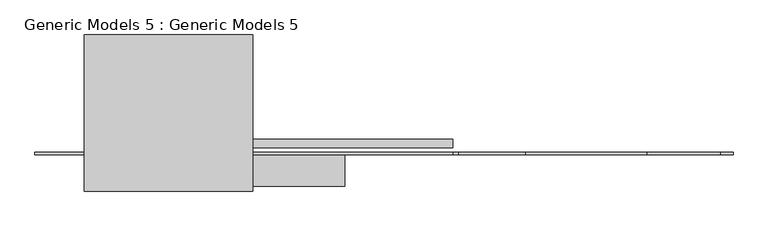
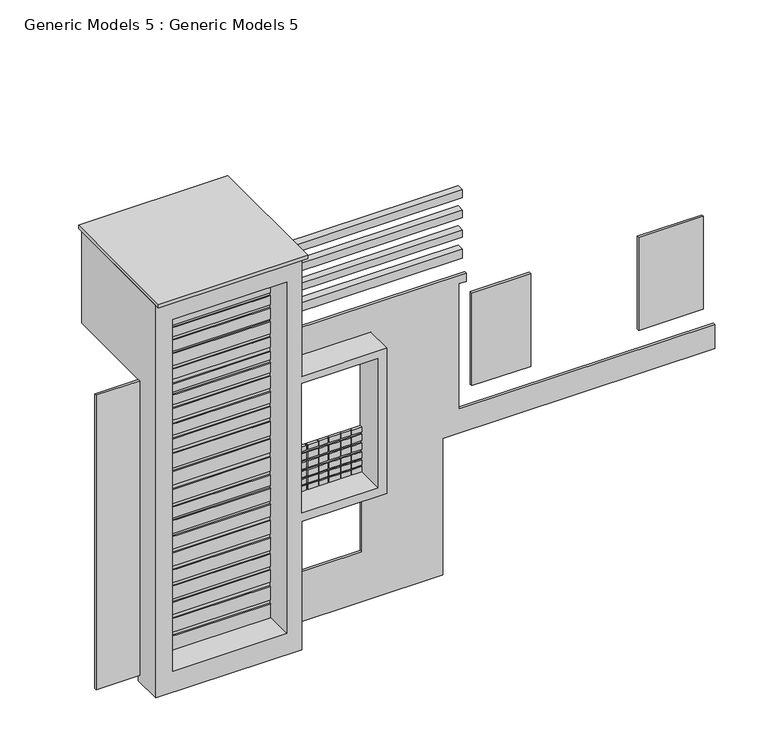
"""IFC4 building model written with IfcOpenShell, lengths in millimetres: proxy geometry, Generic Models 5 : Generic Models 5."""

from ifc_helpers import new_model, si_unit, frame, origin, place, context, project, spatial, polyline, outline, extrude, faceted_brep, source, transform, mapped, element, save


def generic_models_5_generic_models_5_751a22c3(model_context):
    return source(origin(), model_context, "Body", "SolidModel", [
        extrude(outline(polyline([(-4031.0859258, -11851.8777232), (-5326.4859258, -11851.8777232), (-5326.4859258, -11801.0777232), (-4031.0859258, -11801.0777232), (-4031.0859258, -11851.8777232)])), frame((0.0, 0.0, 3959.8880455), z_axis=(0.0, 0.0, 1.0), x_axis=(1.0, 0.0, 0.0)), (0.0, 0.0, 1.0), 1974.0451783),
        extrude(outline(polyline([(-7498.1859258, -11851.8777232), (-8679.2859258, -11851.8777232), (-8679.2859258, -11801.0777232), (-7498.1859258, -11801.0777232), (-7498.1859258, -11851.8777232)])), frame((0.0, 0.0, 3961.5542172), z_axis=(0.0, 0.0, 1.0), x_axis=(1.0, 0.0, 0.0)), (0.0, 0.0, 1.0), 1972.3790066),
        faceted_brep([(-12413.0859258, -11851.8777232, 3860.2469154), (-12413.0859258, -11851.8777232, 3758.0237467), (-12212.1386934, -11851.8777232, 3758.0237467), (-12212.1386934, -11851.8777232, 3860.2469154), (-12413.0859258, -11851.8777232, 3705.6018862), (-12413.0859258, -11851.8777232, 3567.9945022), (-12212.1386934, -11851.8777232, 3567.9945022), (-12212.1386934, -11851.8777232, 3705.6018862), (-12413.0859258, -11851.8777232, 3518.8490079), (-12413.0859258, -11851.8777232, 3383.7067756), (-12212.1386934, -11851.8777232, 3383.7067756), (-12212.1386934, -11851.8777232, 3518.8490079), (-12413.0859258, -11851.8777232, 3332.0961296), (-12413.0859258, -11851.8777232, 3204.3178444), (-12212.1386934, -11851.8777232, 3204.3178444), (-12212.1386934, -11851.8777232, 3332.0961296), (-12413.0859258, -11851.8777232, 3015.7193284), (-12413.0859258, -11851.8777232, 2907.1666358), (-12212.1386934, -11851.8777232, 2907.1666358), (-12212.1386934, -11851.8777232, 3015.7193284), (-12413.0859258, -11851.8777232, 3163.365824), (-12413.0859258, -11851.8777232, 3048.0), (-12212.1386934, -11851.8777232, 3048.0), (-12212.1386934, -11851.8777232, 3163.365824), (-10889.0859258, -11851.8777232, 3758.0237467), (-10889.0859258, -11851.8777232, 3860.2469154), (-11089.7671408, -11851.8777232, 3860.2469154), (-11089.7671408, -11851.8777232, 3758.0237467), (-10889.0859258, -11851.8777232, 3567.9945022), (-10889.0859258, -11851.8777232, 3705.6018862), (-11089.7671408, -11851.8777232, 3705.6018862), (-11089.7671408, -11851.8777232, 3567.9945022), (-10889.0859258, -11851.8777232, 3383.7067756), (-10889.0859258, -11851.8777232, 3518.8490079), (-11089.7671408, -11851.8777232, 3518.8490079), (-11089.7671408, -11851.8777232, 3383.7067756), (-10889.0859258, -11851.8777232, 3204.3178444), (-10889.0859258, -11851.8777232, 3332.0961296), (-11089.7671408, -11851.8777232, 3332.0961296), (-11089.7671408, -11851.8777232, 3204.3178444), (-10889.0859258, -11851.8777232, 2907.1666358), (-10889.0859258, -11851.8777232, 3015.7193284), (-11089.7671408, -11851.8777232, 3015.7193284), (-11089.7671408, -11851.8777232, 2907.1666358), (-10889.0859258, -11851.8777232, 3048.0), (-10889.0859258, -11851.8777232, 3163.365824), (-11089.7671408, -11851.8777232, 3163.365824), (-11089.7671408, -11851.8777232, 3048.0), (-11318.1191266, -11851.8777232, 3860.2469154), (-11542.1625843, -11851.8777232, 3860.2469154), (-11542.1625843, -11851.8777232, 3758.0237467), (-11318.1191266, -11851.8777232, 3758.0237467), (-11107.0012529, -11851.8777232, 3860.2469154), (-11300.8850144, -11851.8777232, 3860.2469154), (-11300.8850144, -11851.8777232, 3758.0237467), (-11107.0012529, -11851.8777232, 3758.0237467), (-11568.0137525, -11851.8777232, 3860.2469154), (-11742.5091378, -11851.8777232, 3860.2469154), (-11742.5091378, -11851.8777232, 3758.0237467), (-11568.0137525, -11851.8777232, 3758.0237467), (-11766.206042, -11851.8777232, 3860.2469154), (-11977.3239156, -11851.8777232, 3860.2469154), (-11977.3239156, -11851.8777232, 3758.0237467), (-11766.206042, -11851.8777232, 3758.0237467), (-12005.3293478, -11851.8777232, 3860.2469154), (-12192.7503172, -11851.8777232, 3860.2469154), (-12192.7503172, -11851.8777232, 3758.0237467), (-12005.3293478, -11851.8777232, 3758.0237467), (-11542.1625843, -11851.8777232, 2907.1666358), (-11318.1191266, -11851.8777232, 2907.1666358), (-11318.1191266, -11851.8777232, 3015.7193284), (-11542.1625843, -11851.8777232, 3015.7193284), (-11300.8850144, -11851.8777232, 2907.1666358), (-11107.0012529, -11851.8777232, 2907.1666358), (-11107.0012529, -11851.8777232, 3015.7193284), (-11300.8850144, -11851.8777232, 3015.7193284), (-11742.5091378, -11851.8777232, 2907.1666358), (-11568.0137525, -11851.8777232, 2907.1666358), (-11568.0137525, -11851.8777232, 3015.7193284), (-11742.5091378, -11851.8777232, 3015.7193284), (-11977.3239156, -11851.8777232, 2907.1666358), (-11766.206042, -11851.8777232, 2907.1666358), (-11766.206042, -11851.8777232, 3015.7193284), (-11977.3239156, -11851.8777232, 3015.7193284), (-12192.7503172, -11851.8777232, 2907.1666358), (-12005.3293478, -11851.8777232, 2907.1666358), (-12005.3293478, -11851.8777232, 3015.7193284), (-12192.7503172, -11851.8777232, 3015.7193284), (-11542.1625843, -11851.8777232, 3567.9945022), (-11318.1191266, -11851.8777232, 3567.9945022), (-11318.1191266, -11851.8777232, 3705.6018862), (-11542.1625843, -11851.8777232, 3705.6018862), (-11300.8850144, -11851.8777232, 3567.9945022), (-11107.0012529, -11851.8777232, 3567.9945022), (-11107.0012529, -11851.8777232, 3705.6018862), (-11300.8850144, -11851.8777232, 3705.6018862), (-11742.5091378, -11851.8777232, 3567.9945022), (-11568.0137525, -11851.8777232, 3567.9945022), (-11568.0137525, -11851.8777232, 3705.6018862), (-11742.5091378, -11851.8777232, 3705.6018862), (-11977.3239156, -11851.8777232, 3567.9945022), (-11766.206042, -11851.8777232, 3567.9945022), (-11766.206042, -11851.8777232, 3705.6018862), (-11977.3239156, -11851.8777232, 3705.6018862), (-12192.7503172, -11851.8777232, 3567.9945022), (-12005.3293478, -11851.8777232, 3567.9945022), (-12005.3293478, -11851.8777232, 3705.6018862), (-12192.7503172, -11851.8777232, 3705.6018862), (-11542.1625843, -11851.8777232, 3383.7067756), (-11318.1191266, -11851.8777232, 3383.7067756), (-11318.1191266, -11851.8777232, 3518.8490079), (-11542.1625843, -11851.8777232, 3518.8490079), (-11300.8850144, -11851.8777232, 3383.7067756), (-11107.0012529, -11851.8777232, 3383.7067756), (-11107.0012529, -11851.8777232, 3518.8490079), (-11300.8850144, -11851.8777232, 3518.8490079), (-11742.5091378, -11851.8777232, 3383.7067756), (-11568.0137525, -11851.8777232, 3383.7067756), (-11568.0137525, -11851.8777232, 3518.8490079), (-11742.5091378, -11851.8777232, 3518.8490079), (-11977.3239156, -11851.8777232, 3383.7067756), (-11766.206042, -11851.8777232, 3383.7067756), (-11766.206042, -11851.8777232, 3518.8490079), (-11977.3239156, -11851.8777232, 3518.8490079), (-12192.7503172, -11851.8777232, 3383.7067756), (-12005.3293478, -11851.8777232, 3383.7067756), (-12005.3293478, -11851.8777232, 3518.8490079), (-12192.7503172, -11851.8777232, 3518.8490079), (-11542.1625843, -11851.8777232, 3204.3178444), (-11318.1191266, -11851.8777232, 3204.3178444), (-11318.1191266, -11851.8777232, 3332.0961296), (-11542.1625843, -11851.8777232, 3332.0961296), (-11300.8850144, -11851.8777232, 3204.3178444), (-11107.0012529, -11851.8777232, 3204.3178444), (-11107.0012529, -11851.8777232, 3332.0961296), (-11300.8850144, -11851.8777232, 3332.0961296), (-11742.5091378, -11851.8777232, 3204.3178444), (-11568.0137525, -11851.8777232, 3204.3178444), (-11568.0137525, -11851.8777232, 3332.0961296), (-11742.5091378, -11851.8777232, 3332.0961296), (-11977.3239156, -11851.8777232, 3204.3178444), (-11766.206042, -11851.8777232, 3204.3178444), (-11766.206042, -11851.8777232, 3332.0961296), (-11977.3239156, -11851.8777232, 3332.0961296), (-12192.7503172, -11851.8777232, 3204.3178444), (-12005.3293478, -11851.8777232, 3204.3178444), (-12005.3293478, -11851.8777232, 3332.0961296), (-12192.7503172, -11851.8777232, 3332.0961296), (-11542.1625843, -11851.8777232, 3048.0), (-11318.1191266, -11851.8777232, 3048.0), (-11318.1191266, -11851.8777232, 3163.365824), (-11542.1625843, -11851.8777232, 3163.365824), (-11300.8850144, -11851.8777232, 3048.0), (-11107.0012529, -11851.8777232, 3048.0), (-11107.0012529, -11851.8777232, 3163.365824), (-11300.8850144, -11851.8777232, 3163.365824), (-11742.5091378, -11851.8777232, 3048.0), (-11568.0137525, -11851.8777232, 3048.0), (-11568.0137525, -11851.8777232, 3163.365824), (-11742.5091378, -11851.8777232, 3163.365824), (-11977.3239156, -11851.8777232, 3048.0), (-11766.206042, -11851.8777232, 3048.0), (-11766.206042, -11851.8777232, 3163.365824), (-11977.3239156, -11851.8777232, 3163.365824), (-12192.7503172, -11851.8777232, 3048.0), (-12005.3293478, -11851.8777232, 3048.0), (-12005.3293478, -11851.8777232, 3163.365824), (-12192.7503172, -11851.8777232, 3163.365824), (-10889.0859258, -11801.0777232, 3860.2469154), (-10889.0859258, -11801.0777232, 2907.1666358), (-12413.0859258, -11801.0777232, 2907.1666358), (-12413.0859258, -11801.0777232, 3860.2469154), (-12212.1386934, -11826.4777232, 3860.2469154), (-12192.7503172, -11826.4777232, 3860.2469154), (-12005.3293478, -11826.4777232, 3860.2469154), (-11977.3239156, -11826.4777232, 3860.2469154), (-11766.206042, -11826.4777232, 3860.2469154), (-11742.5091378, -11826.4777232, 3860.2469154), (-11568.0137525, -11826.4777232, 3860.2469154), (-11542.1625843, -11826.4777232, 3860.2469154), (-11318.1191266, -11826.4777232, 3860.2469154), (-11300.8850144, -11826.4777232, 3860.2469154), (-11107.0012529, -11826.4777232, 3860.2469154), (-11089.7671408, -11826.4777232, 3860.2469154), (-12413.0859258, -11826.4777232, 3015.7193284), (-12413.0859258, -11826.4777232, 3048.0), (-12413.0859258, -11826.4777232, 3163.365824), (-12413.0859258, -11826.4777232, 3204.3178444), (-12413.0859258, -11826.4777232, 3332.0961296), (-12413.0859258, -11826.4777232, 3383.7067756), (-12413.0859258, -11826.4777232, 3518.8490079), (-12413.0859258, -11826.4777232, 3567.9945022), (-12413.0859258, -11826.4777232, 3705.6018862), (-12413.0859258, -11826.4777232, 3758.0237467), (-11089.7671408, -11826.4777232, 2907.1666358), (-11107.0012529, -11826.4777232, 2907.1666358), (-11300.8850144, -11826.4777232, 2907.1666358), (-11318.1191266, -11826.4777232, 2907.1666358), (-11542.1625843, -11826.4777232, 2907.1666358), (-11568.0137525, -11826.4777232, 2907.1666358), (-11742.5091378, -11826.4777232, 2907.1666358), (-11766.206042, -11826.4777232, 2907.1666358), (-11977.3239156, -11826.4777232, 2907.1666358), (-12005.3293478, -11826.4777232, 2907.1666358), (-12192.7503172, -11826.4777232, 2907.1666358), (-12212.1386934, -11826.4777232, 2907.1666358), (-10889.0859258, -11826.4777232, 3758.0237467), (-10889.0859258, -11826.4777232, 3705.6018862), (-10889.0859258, -11826.4777232, 3567.9945022), (-10889.0859258, -11826.4777232, 3518.8490079), (-10889.0859258, -11826.4777232, 3383.7067756), (-10889.0859258, -11826.4777232, 3332.0961296), (-10889.0859258, -11826.4777232, 3204.3178444), (-10889.0859258, -11826.4777232, 3163.365824), (-10889.0859258, -11826.4777232, 3048.0), (-10889.0859258, -11826.4777232, 3015.7193284), (-12212.1386934, -11826.4777232, 3705.6018862), (-12212.1386934, -11826.4777232, 3567.9945022), (-12212.1386934, -11826.4777232, 3518.8490079), (-12212.1386934, -11826.4777232, 3383.7067756), (-12212.1386934, -11826.4777232, 3332.0961296), (-12212.1386934, -11826.4777232, 3204.3178444), (-12212.1386934, -11826.4777232, 3163.365824), (-12212.1386934, -11826.4777232, 3048.0), (-12212.1386934, -11826.4777232, 3015.7193284), (-12192.7503172, -11826.4777232, 3015.7193284), (-12005.3293478, -11826.4777232, 3015.7193284), (-11977.3239156, -11826.4777232, 3015.7193284), (-11766.206042, -11826.4777232, 3015.7193284), (-11742.5091378, -11826.4777232, 3015.7193284), (-11568.0137525, -11826.4777232, 3015.7193284), (-11542.1625843, -11826.4777232, 3015.7193284), (-11318.1191266, -11826.4777232, 3015.7193284), (-11300.8850144, -11826.4777232, 3015.7193284), (-11107.0012529, -11826.4777232, 3015.7193284), (-11089.7671408, -11826.4777232, 3015.7193284), (-11089.7671408, -11826.4777232, 3048.0), (-11089.7671408, -11826.4777232, 3163.365824), (-11089.7671408, -11826.4777232, 3204.3178444), (-11089.7671408, -11826.4777232, 3332.0961296), (-11089.7671408, -11826.4777232, 3383.7067756), (-11089.7671408, -11826.4777232, 3518.8490079), (-11089.7671408, -11826.4777232, 3567.9945022), (-11089.7671408, -11826.4777232, 3705.6018862), (-11089.7671408, -11826.4777232, 3758.0237467), (-11107.0012529, -11826.4777232, 3758.0237467), (-11300.8850144, -11826.4777232, 3758.0237467), (-11318.1191266, -11826.4777232, 3758.0237467), (-11542.1625843, -11826.4777232, 3758.0237467), (-11568.0137525, -11826.4777232, 3758.0237467), (-11742.5091378, -11826.4777232, 3758.0237467), (-11766.206042, -11826.4777232, 3758.0237467), (-11977.3239156, -11826.4777232, 3758.0237467), (-12005.3293478, -11826.4777232, 3758.0237467), (-12192.7503172, -11826.4777232, 3758.0237467), (-12212.1386934, -11826.4777232, 3758.0237467), (-11542.1625843, -11826.4777232, 3705.6018862), (-11318.1191266, -11826.4777232, 3705.6018862), (-11318.1191266, -11826.4777232, 3567.9945022), (-11542.1625843, -11826.4777232, 3567.9945022), (-11300.8850144, -11826.4777232, 3705.6018862), (-11107.0012529, -11826.4777232, 3705.6018862), (-11107.0012529, -11826.4777232, 3567.9945022), (-11300.8850144, -11826.4777232, 3567.9945022), (-11742.5091378, -11826.4777232, 3705.6018862), (-11568.0137525, -11826.4777232, 3705.6018862), (-11568.0137525, -11826.4777232, 3567.9945022), (-11742.5091378, -11826.4777232, 3567.9945022), (-11977.3239156, -11826.4777232, 3705.6018862), (-11766.206042, -11826.4777232, 3705.6018862), (-11766.206042, -11826.4777232, 3567.9945022), (-11977.3239156, -11826.4777232, 3567.9945022), (-12192.7503172, -11826.4777232, 3705.6018862), (-12005.3293478, -11826.4777232, 3705.6018862), (-12005.3293478, -11826.4777232, 3567.9945022), (-12192.7503172, -11826.4777232, 3567.9945022), (-11542.1625843, -11826.4777232, 3518.8490079), (-11318.1191266, -11826.4777232, 3518.8490079), (-11318.1191266, -11826.4777232, 3383.7067756), (-11542.1625843, -11826.4777232, 3383.7067756), (-11300.8850144, -11826.4777232, 3518.8490079), (-11107.0012529, -11826.4777232, 3518.8490079), (-11107.0012529, -11826.4777232, 3383.7067756), (-11300.8850144, -11826.4777232, 3383.7067756), (-11742.5091378, -11826.4777232, 3518.8490079), (-11568.0137525, -11826.4777232, 3518.8490079), (-11568.0137525, -11826.4777232, 3383.7067756), (-11742.5091378, -11826.4777232, 3383.7067756), (-11977.3239156, -11826.4777232, 3518.8490079), (-11766.206042, -11826.4777232, 3518.8490079), (-11766.206042, -11826.4777232, 3383.7067756), (-11977.3239156, -11826.4777232, 3383.7067756), (-12192.7503172, -11826.4777232, 3518.8490079), (-12005.3293478, -11826.4777232, 3518.8490079), (-12005.3293478, -11826.4777232, 3383.7067756), (-12192.7503172, -11826.4777232, 3383.7067756), (-11542.1625843, -11826.4777232, 3332.0961296), (-11318.1191266, -11826.4777232, 3332.0961296), (-11318.1191266, -11826.4777232, 3204.3178444), (-11542.1625843, -11826.4777232, 3204.3178444), (-11300.8850144, -11826.4777232, 3332.0961296), (-11107.0012529, -11826.4777232, 3332.0961296), (-11107.0012529, -11826.4777232, 3204.3178444), (-11300.8850144, -11826.4777232, 3204.3178444), (-11742.5091378, -11826.4777232, 3332.0961296), (-11568.0137525, -11826.4777232, 3332.0961296), (-11568.0137525, -11826.4777232, 3204.3178444), (-11742.5091378, -11826.4777232, 3204.3178444), (-11977.3239156, -11826.4777232, 3332.0961296), (-11766.206042, -11826.4777232, 3332.0961296), (-11766.206042, -11826.4777232, 3204.3178444), (-11977.3239156, -11826.4777232, 3204.3178444), (-12192.7503172, -11826.4777232, 3332.0961296), (-12005.3293478, -11826.4777232, 3332.0961296), (-12005.3293478, -11826.4777232, 3204.3178444), (-12192.7503172, -11826.4777232, 3204.3178444), (-11542.1625843, -11826.4777232, 3163.365824), (-11318.1191266, -11826.4777232, 3163.365824), (-11318.1191266, -11826.4777232, 3048.0), (-11542.1625843, -11826.4777232, 3048.0), (-11300.8850144, -11826.4777232, 3163.365824), (-11107.0012529, -11826.4777232, 3163.365824), (-11107.0012529, -11826.4777232, 3048.0), (-11300.8850144, -11826.4777232, 3048.0), (-11742.5091378, -11826.4777232, 3163.365824), (-11568.0137525, -11826.4777232, 3163.365824), (-11568.0137525, -11826.4777232, 3048.0), (-11742.5091378, -11826.4777232, 3048.0), (-11977.3239156, -11826.4777232, 3163.365824), (-11766.206042, -11826.4777232, 3163.365824), (-11766.206042, -11826.4777232, 3048.0), (-11977.3239156, -11826.4777232, 3048.0), (-12192.7503172, -11826.4777232, 3163.365824), (-12005.3293478, -11826.4777232, 3163.365824), (-12005.3293478, -11826.4777232, 3048.0), (-12192.7503172, -11826.4777232, 3048.0)], [[[0, 1, 2, 3]], [[4, 5, 6, 7]], [[8, 9, 10, 11]], [[12, 13, 14, 15]], [[16, 17, 18, 19]], [[20, 21, 22, 23]], [[24, 25, 26, 27]], [[28, 29, 30, 31]], [[32, 33, 34, 35]], [[36, 37, 38, 39]], [[40, 41, 42, 43]], [[44, 45, 46, 47]], [[48, 49, 50, 51]], [[52, 53, 54, 55]], [[56, 57, 58, 59]], [[60, 61, 62, 63]], [[64, 65, 66, 67]], [[68, 69, 70, 71]], [[72, 73, 74, 75]], [[76, 77, 78, 79]], [[80, 81, 82, 83]], [[84, 85, 86, 87]], [[88, 89, 90, 91]], [[92, 93, 94, 95]], [[96, 97, 98, 99]], [[100, 101, 102, 103]], [[104, 105, 106, 107]], [[108, 109, 110, 111]], [[112, 113, 114, 115]], [[116, 117, 118, 119]], [[120, 121, 122, 123]], [[124, 125, 126, 127]], [[128, 129, 130, 131]], [[132, 133, 134, 135]], [[136, 137, 138, 139]], [[140, 141, 142, 143]], [[144, 145, 146, 147]], [[148, 149, 150, 151]], [[152, 153, 154, 155]], [[156, 157, 158, 159]], [[160, 161, 162, 163]], [[164, 165, 166, 167]], [[168, 169, 170, 171]], [[168, 171, 0, 3, 172, 173, 65, 64, 174, 175, 61, 60, 176, 177, 57, 56, 178, 179, 49, 48, 180, 181, 53, 52, 182, 183, 26, 25]], [[171, 170, 17, 16, 184, 185, 21, 20, 186, 187, 13, 12, 188, 189, 9, 8, 190, 191, 5, 4, 192, 193, 1, 0]], [[170, 169, 40, 43, 194, 195, 73, 72, 196, 197, 69, 68, 198, 199, 77, 76, 200, 201, 81, 80, 202, 203, 85, 84, 204, 205, 18, 17]], [[169, 168, 25, 24, 206, 207, 29, 28, 208, 209, 33, 32, 210, 211, 37, 36, 212, 213, 45, 44, 214, 215, 41, 40]], [[193, 192, 216, 217, 191, 190, 218, 219, 189, 188, 220, 221, 187, 186, 222, 223, 185, 184, 224, 205, 204, 225, 226, 203, 202, 227, 228, 201, 200, 229, 230, 199, 198, 231, 232, 197, 196, 233, 234, 195, 194, 235, 215, 214, 236, 237, 213, 212, 238, 239, 211, 210, 240, 241, 209, 208, 242, 243, 207, 206, 244, 183, 182, 245, 246, 181, 180, 247, 248, 179, 178, 249, 250, 177, 176, 251, 252, 175, 174, 253, 254, 173, 172, 255], [256, 257, 258, 259], [260, 261, 262, 263], [264, 265, 266, 267], [268, 269, 270, 271], [272, 273, 274, 275], [276, 277, 278, 279], [280, 281, 282, 283], [284, 285, 286, 287], [288, 289, 290, 291], [292, 293, 294, 295], [296, 297, 298, 299], [300, 301, 302, 303], [304, 305, 306, 307], [308, 309, 310, 311], [312, 313, 314, 315], [316, 317, 318, 319], [320, 321, 322, 323], [324, 325, 326, 327], [328, 329, 330, 331], [332, 333, 334, 335]], [[91, 90, 257, 256]], [[95, 94, 261, 260]], [[99, 98, 265, 264]], [[103, 102, 269, 268]], [[107, 106, 273, 272]], [[192, 4, 7, 216]], [[29, 207, 243, 30]], [[51, 50, 248, 247]], [[55, 54, 246, 245]], [[59, 58, 250, 249]], [[63, 62, 252, 251]], [[67, 66, 254, 253]], [[1, 193, 255, 2]], [[206, 24, 27, 244]], [[111, 110, 277, 276]], [[115, 114, 281, 280]], [[119, 118, 285, 284]], [[123, 122, 289, 288]], [[127, 126, 293, 292]], [[190, 8, 11, 218]], [[33, 209, 241, 34]], [[89, 88, 259, 258]], [[93, 92, 263, 262]], [[97, 96, 267, 266]], [[101, 100, 271, 270]], [[105, 104, 275, 274]], [[5, 191, 217, 6]], [[208, 28, 31, 242]], [[131, 130, 297, 296]], [[135, 134, 301, 300]], [[139, 138, 305, 304]], [[143, 142, 309, 308]], [[147, 146, 313, 312]], [[188, 12, 15, 220]], [[37, 211, 239, 38]], [[109, 108, 279, 278]], [[113, 112, 283, 282]], [[117, 116, 287, 286]], [[121, 120, 291, 290]], [[125, 124, 295, 294]], [[9, 189, 219, 10]], [[210, 32, 35, 240]], [[151, 150, 317, 316]], [[155, 154, 321, 320]], [[159, 158, 325, 324]], [[163, 162, 329, 328]], [[167, 166, 333, 332]], [[186, 20, 23, 222]], [[45, 213, 237, 46]], [[129, 128, 299, 298]], [[133, 132, 303, 302]], [[137, 136, 307, 306]], [[141, 140, 311, 310]], [[145, 144, 315, 314]], [[13, 187, 221, 14]], [[212, 36, 39, 238]], [[71, 70, 232, 231]], [[75, 74, 234, 233]], [[79, 78, 230, 229]], [[83, 82, 228, 227]], [[87, 86, 226, 225]], [[184, 16, 19, 224]], [[41, 215, 235, 42]], [[149, 148, 319, 318]], [[153, 152, 323, 322]], [[157, 156, 327, 326]], [[161, 160, 331, 330]], [[165, 164, 335, 334]], [[21, 185, 223, 22]], [[214, 44, 47, 236]], [[231, 198, 68, 71]], [[179, 248, 50, 49]], [[256, 259, 88, 91]], [[276, 279, 108, 111]], [[296, 299, 128, 131]], [[316, 319, 148, 151]], [[199, 230, 78, 77]], [[249, 178, 56, 59]], [[266, 265, 98, 97]], [[286, 285, 118, 117]], [[306, 305, 138, 137]], [[326, 325, 158, 157]], [[233, 196, 72, 75]], [[181, 246, 54, 53]], [[260, 263, 92, 95]], [[280, 283, 112, 115]], [[300, 303, 132, 135]], [[320, 323, 152, 155]], [[197, 232, 70, 69]], [[247, 180, 48, 51]], [[258, 257, 90, 89]], [[278, 277, 110, 109]], [[298, 297, 130, 129]], [[318, 317, 150, 149]], [[235, 194, 43, 42]], [[237, 236, 47, 46]], [[239, 238, 39, 38]], [[241, 240, 35, 34]], [[243, 242, 31, 30]], [[183, 244, 27, 26]], [[195, 234, 74, 73]], [[245, 182, 52, 55]], [[262, 261, 94, 93]], [[282, 281, 114, 113]], [[302, 301, 134, 133]], [[322, 321, 154, 153]], [[229, 200, 76, 79]], [[177, 250, 58, 57]], [[264, 267, 96, 99]], [[284, 287, 116, 119]], [[304, 307, 136, 139]], [[324, 327, 156, 159]], [[201, 228, 82, 81]], [[251, 176, 60, 63]], [[270, 269, 102, 101]], [[290, 289, 122, 121]], [[310, 309, 142, 141]], [[330, 329, 162, 161]], [[227, 202, 80, 83]], [[175, 252, 62, 61]], [[268, 271, 100, 103]], [[288, 291, 120, 123]], [[308, 311, 140, 143]], [[328, 331, 160, 163]], [[203, 226, 86, 85]], [[253, 174, 64, 67]], [[274, 273, 106, 105]], [[294, 293, 126, 125]], [[314, 313, 146, 145]], [[334, 333, 166, 165]], [[225, 204, 84, 87]], [[173, 254, 66, 65]], [[272, 275, 104, 107]], [[292, 295, 124, 127]], [[312, 315, 144, 147]], [[332, 335, 164, 167]], [[217, 216, 7, 6]], [[219, 218, 11, 10]], [[221, 220, 15, 14]], [[223, 222, 23, 22]], [[205, 224, 19, 18]], [[255, 172, 3, 2]]]),
        extrude(outline(polyline([(-15345.7421486, -11851.8777232), (-16223.0859258, -11851.8777232), (-16223.0859258, -11801.0777232), (-15345.7421486, -11801.0777232), (-15345.7421486, -11851.8777232)])), frame((0.0, 0.0, 146.3632195), z_axis=(0.0, 0.0, 1.0), x_axis=(1.0, 0.0, 0.0)), (0.0, 0.0, 1.0), 6254.4367805),
        faceted_brep([(-8937.544821, -11851.8777232, 6219.2721294), (-8793.5859258, -11851.8777232, 6219.2721294), (-8793.5859258, -11851.8777232, 6400.8), (-12413.0859258, -11851.8777232, 6400.8), (-12413.0859258, -11851.8777232, 5813.3511684), (-10711.2859258, -11851.8777232, 5813.3511684), (-10711.2859258, -11851.8777232, 2726.819022), (-10889.0859258, -11851.8777232, 2726.819022), (-10889.0859258, -11851.8777232, 1204.6732896), (-12413.0859258, -11851.8777232, 1204.6732896), (-12413.0859258, -11851.8777232, 146.3632195), (-9263.4859258, -11851.8777232, 146.3632195), (-9263.4859258, -11851.8777232, 3048.0), (-3802.4859258, -11851.8777232, 3048.0), (-3802.4859258, -11851.8777232, 3555.4469154), (-8937.5521993, -11851.8777232, 3555.4469154), (-8793.5859258, -11801.0777232, 6400.8), (-8793.5859258, -11801.0777232, 6219.2721294), (-8937.544821, -11801.0777232, 6219.2721294), (-8937.5510186, -11801.0777232, 3555.4469154), (-3802.4859258, -11801.0777232, 3555.4469154), (-3802.4859258, -11801.0777232, 3048.0), (-9263.4859258, -11801.0777232, 3048.0), (-9263.4859258, -11801.0777232, 146.3632195), (-12413.0859258, -11801.0777232, 146.3632195), (-12413.0859258, -11801.0777232, 1204.6732896), (-10889.0859258, -11801.0777232, 1204.6732896), (-10889.0859258, -11801.0777232, 2726.819022), (-10711.2859258, -11801.0777232, 2726.819022), (-10711.2859258, -11801.0777232, 5813.3511684), (-12413.0859258, -11801.0777232, 5813.3511684), (-12413.0859258, -11801.0777232, 6400.8)], [[[0, 1, 2, 3, 4, 5, 6, 7, 8, 9, 10, 11, 12, 13, 14, 15]], [[16, 17, 18, 19, 20, 21, 22, 23, 24, 25, 26, 27, 28, 29, 30, 31]], [[2, 16, 31, 3]], [[1, 0, 18, 17]], [[2, 1, 17, 16]], [[4, 3, 31, 30]], [[4, 30, 29, 5]], [[18, 0, 15, 19]], [[5, 29, 28, 6]], [[21, 13, 12, 22]], [[14, 13, 21, 20]], [[15, 14, 20, 19]], [[24, 23, 11, 10]], [[12, 11, 23, 22]], [[7, 6, 28, 27]], [[7, 27, 26, 8]], [[9, 8, 26, 25]], [[10, 9, 25, 24]]]),
        extrude(outline(polyline([(-12348.5421486, -12495.260612), (-15345.7421486, -12495.260612), (-15345.7421486, -9718.2777232), (-12348.5421486, -9718.2777232), (-12348.5421486, -12495.260612)])), frame((0.0, 0.0, 8339.6495124), z_axis=(0.0, 0.0, 1.0), x_axis=(1.0, 0.0, 0.0)), (0.0, 0.0, 1.0), 76.2),
        extrude(outline(polyline([(-12413.0859258, -11724.8777232), (-12413.0859258, -11572.4777232), (-8793.5859258, -11572.4777232), (-8793.5859258, -11724.8777232), (-12413.0859258, -11724.8777232)])), frame((0.0, 0.0, 7921.1981314), z_axis=(0.0, 0.0, 1.0), x_axis=(1.0, 0.0, 0.0)), (0.0, 0.0, 1.0), 166.2555086),
        extrude(outline(polyline([(-12413.0859258, -11724.8777232), (-12413.0859258, -11572.4777232), (-8793.5859258, -11572.4777232), (-8793.5859258, -11724.8777232), (-12413.0859258, -11724.8777232)])), frame((0.0, 0.0, 7497.682031), z_axis=(0.0, 0.0, 1.0), x_axis=(1.0, 0.0, 0.0)), (0.0, 0.0, 1.0), 158.2780216),
        extrude(outline(polyline([(-12413.0859258, -11724.8777232), (-12413.0859258, -11572.4777232), (-8793.5859258, -11572.4777232), (-8793.5859258, -11724.8777232), (-12413.0859258, -11724.8777232)])), frame((0.0, 0.0, 7084.7958383), z_axis=(0.0, 0.0, 1.0), x_axis=(1.0, 0.0, 0.0)), (0.0, 0.0, 1.0), 146.1467071),
        extrude(outline(polyline([(-12413.0859258, -11724.8777232), (-12413.0859258, -11572.4777232), (-8793.5859258, -11572.4777232), (-8793.5859258, -11724.8777232), (-12413.0859258, -11724.8777232)])), frame((0.0, 0.0, 6637.6676542), z_axis=(0.0, 0.0, 1.0), x_axis=(1.0, 0.0, 0.0)), (0.0, 0.0, 1.0), 186.6390803),
        faceted_brep([(-12413.0859258, -9819.8777232, 8339.6495124), (-15345.7421486, -9819.8777232, 8339.6495124), (-15345.7421486, -12410.6777232, 8339.6495124), (-12413.0859258, -12410.6777232, 8339.6495124), (-15345.7421486, -11801.0777232, 6400.8), (-15345.7421486, -9819.8777232, 6400.8), (-12413.0859258, -9819.8777232, 6400.8), (-12413.0859258, -11801.0777232, 6400.8), (-12413.0859258, -12410.6777232, 5809.1140305), (-12413.0859258, -11801.0777232, 5809.1140305), (-12413.0859258, -12410.6777232, 0.0), (-12413.0859258, -11801.0777232, 0.0), (-12413.0859258, -11801.0777232, 2726.819022), (-12413.0859258, -12410.6777232, 2726.819022), (-12413.0859258, -12410.6777232, 5656.7140305), (-12413.0859258, -12410.6777232, 2907.1666358), (-12413.0859258, -11801.0777232, 2907.1666358), (-12413.0859258, -11801.0777232, 5656.7140305), (-15345.7421486, -11801.0777232, 0.0), (-15345.7421486, -12410.6777232, 0.0), (-10711.2859258, -12410.6777232, 2726.819022), (-10711.2859258, -12410.6777232, 5809.1140305), (-12719.9872036, -12410.6777232, 449.1643292), (-15005.9872036, -12410.6777232, 449.1643292), (-15005.9872036, -12410.6777232, 7921.1981314), (-12719.9872036, -12410.6777232, 7921.1981314), (-10889.0859258, -12410.6777232, 2907.1666358), (-10889.0859258, -12410.6777232, 5656.7140305), (-10711.2859258, -11801.0777232, 5809.1140305), (-10711.2859258, -11801.0777232, 2726.819022), (-10889.0859258, -11801.0777232, 2907.1666358), (-10889.0859258, -11801.0777232, 5656.7140305), (-12719.9872036, -11851.8777232, 7921.1981314), (-15005.9872036, -11851.8777232, 7921.1981314), (-15005.9872036, -11851.8777232, 7641.4779552), (-12719.9872036, -11851.8777232, 7641.4779552), (-15005.9872036, -11851.8777232, 449.1643292), (-12719.9872036, -11851.8777232, 449.1643292), (-12719.9872036, -11851.8777232, 746.0806359), (-15005.9872036, -11851.8777232, 746.0806359), (-15005.9872036, -11851.8777232, 5579.3149047), (-15005.9872036, -11851.8777232, 5327.1779598), (-12719.9872036, -11851.8777232, 5327.1779598), (-12719.9872036, -11851.8777232, 5579.3149047), (-15005.9872036, -11851.8777232, 5246.9525683), (-15005.9872036, -11851.8777232, 5012.0067787), (-12719.9872036, -11851.8777232, 5012.0067787), (-12719.9872036, -11851.8777232, 5246.9525683), (-15005.9872036, -11851.8777232, 4930.9456759), (-15005.9872036, -11851.8777232, 4701.7302714), (-12719.9872036, -11851.8777232, 4701.7302714), (-12719.9872036, -11851.8777232, 4930.9456759), (-15005.9872036, -11851.8777232, 4617.0202306), (-15005.9872036, -11851.8777232, 4318.0436161), (-12719.9872036, -11851.8777232, 4318.0436161), (-12719.9872036, -11851.8777232, 4617.0202306), (-15005.9872036, -11851.8777232, 5864.0560227), (-15005.9872036, -11851.8777232, 5656.7140305), (-12719.9872036, -11851.8777232, 5656.7140305), (-12719.9872036, -11851.8777232, 5809.1140305), (-12719.9872036, -11851.8777232, 5864.0560227), (-15005.9872036, -11851.8777232, 6100.852455), (-15005.9872036, -11851.8777232, 5929.0509389), (-12719.9872036, -11851.8777232, 5929.0509389), (-12719.9872036, -11851.8777232, 6100.852455), (-15005.9872036, -11851.8777232, 6410.0133188), (-15005.9872036, -11851.8777232, 6202.029587), (-12719.9872036, -11851.8777232, 6202.029587), (-12719.9872036, -11851.8777232, 6410.0133188), (-15005.9872036, -11851.8777232, 6742.3790133), (-15005.9872036, -11851.8777232, 6488.0072182), (-12719.9872036, -11851.8777232, 6488.0072182), (-12719.9872036, -11851.8777232, 6742.3790133), (-15005.9872036, -11851.8777232, 7028.3267483), (-15005.9872036, -11851.8777232, 6794.4813213), (-12719.9872036, -11851.8777232, 6794.4813213), (-12719.9872036, -11851.8777232, 7028.3267483), (-15005.9872036, -11851.8777232, 7291.9244634), (-15005.9872036, -11851.8777232, 7102.8217548), (-12719.9872036, -11851.8777232, 7102.8217548), (-12719.9872036, -11851.8777232, 7291.9244634), (-15005.9872036, -11851.8777232, 7584.1741041), (-15005.9872036, -11851.8777232, 7354.9586997), (-12719.9872036, -11851.8777232, 7354.9586997), (-12719.9872036, -11851.8777232, 7584.1741041), (-15005.9872036, -11851.8777232, 4243.2994625), (-15005.9872036, -11851.8777232, 3957.1268478), (-12719.9872036, -11851.8777232, 3957.1268478), (-12719.9872036, -11851.8777232, 4243.2994625), (-15005.9872036, -11851.8777232, 3860.2469154), (-15005.9872036, -11851.8777232, 3561.7302751), (-12719.9872036, -11851.8777232, 3561.7302751), (-12719.9872036, -11851.8777232, 3860.2469154), (-15005.9872036, -11851.8777232, 3481.7166587), (-15005.9872036, -11851.8777232, 3252.5012542), (-12719.9872036, -11851.8777232, 3252.5012542), (-12719.9872036, -11851.8777232, 3481.7166587), (-15005.9872036, -11851.8777232, 3197.6888749), (-15005.9872036, -11851.8777232, 2923.6269782), (-12719.9872036, -11851.8777232, 2923.6269782), (-12719.9872036, -11851.8777232, 3197.6888749), (-15005.9872036, -11851.8777232, 2858.8487118), (-15005.9872036, -11851.8777232, 2594.7527023), (-12719.9872036, -11851.8777232, 2594.7527023), (-12719.9872036, -11851.8777232, 2858.8487118), (-15005.9872036, -11851.8777232, 2510.0426615), (-15005.9872036, -11851.8777232, 2230.9978213), (-12719.9872036, -11851.8777232, 2230.9978213), (-12719.9872036, -11851.8777232, 2510.0426615), (-15005.9872036, -11851.8777232, 2146.2877805), (-15005.9872036, -11851.8777232, 1882.191771), (-12719.9872036, -11851.8777232, 1882.191771), (-12719.9872036, -11851.8777232, 2146.2877805), (-15005.9872036, -11851.8777232, 1802.4646738), (-15005.9872036, -11851.8777232, 1533.3857208), (-12719.9872036, -11851.8777232, 1533.3857208), (-12719.9872036, -11851.8777232, 1802.4646738), (-15005.9872036, -11851.8777232, 1458.6415671), (-15005.9872036, -11851.8777232, 1204.6732896), (-12719.9872036, -11851.8777232, 1204.6732896), (-12719.9872036, -11851.8777232, 1458.6415671), (-15005.9872036, -11851.8777232, 1114.8184605), (-15005.9872036, -11851.8777232, 825.8077331), (-12719.9872036, -11851.8777232, 825.8077331), (-12719.9872036, -11851.8777232, 1114.8184605), (-12719.9872036, -11826.4777232, 7641.4779552), (-12719.9872036, -11826.4777232, 7584.1741041), (-12719.9872036, -11826.4777232, 7354.9586997), (-12719.9872036, -11826.4777232, 7291.9244634), (-12719.9872036, -11826.4777232, 7102.8217548), (-12719.9872036, -11826.4777232, 7028.3267483), (-12719.9872036, -11826.4777232, 6794.4813213), (-12719.9872036, -11826.4777232, 6742.3790133), (-12719.9872036, -11826.4777232, 6488.0072182), (-12719.9872036, -11826.4777232, 6410.0133188), (-12719.9872036, -11826.4777232, 6202.029587), (-12719.9872036, -11826.4777232, 6100.852455), (-12719.9872036, -11826.4777232, 5929.0509389), (-12719.9872036, -11826.4777232, 5864.0560227), (-12719.9872036, -11826.4777232, 5656.7140305), (-12719.9872036, -11826.4777232, 5579.3149047), (-12719.9872036, -11826.4777232, 5327.1779598), (-12719.9872036, -11826.4777232, 5246.9525683), (-12719.9872036, -11826.4777232, 5012.0067787), (-12719.9872036, -11826.4777232, 4930.9456759), (-12719.9872036, -11826.4777232, 4701.7302714), (-12719.9872036, -11826.4777232, 4617.0202306), (-12719.9872036, -11826.4777232, 4318.0436161), (-12719.9872036, -11826.4777232, 4243.2994625), (-12719.9872036, -11826.4777232, 3957.1268478), (-12719.9872036, -11826.4777232, 3860.2469154), (-12719.9872036, -11826.4777232, 3561.7302751), (-12719.9872036, -11826.4777232, 3481.7166587), (-12719.9872036, -11826.4777232, 3252.5012542), (-12719.9872036, -11826.4777232, 3197.6888749), (-12719.9872036, -11826.4777232, 2923.6269782), (-12719.9872036, -11826.4777232, 2858.8487118), (-12719.9872036, -11826.4777232, 2594.7527023), (-12719.9872036, -11826.4777232, 2510.0426615), (-12719.9872036, -11826.4777232, 2230.9978213), (-12719.9872036, -11826.4777232, 2146.2877805), (-12719.9872036, -11826.4777232, 1882.191771), (-12719.9872036, -11826.4777232, 1802.4646738), (-12719.9872036, -11826.4777232, 1533.3857208), (-12719.9872036, -11826.4777232, 1458.6415671), (-12719.9872036, -11826.4777232, 1204.6732896), (-12719.9872036, -11826.4777232, 1114.8184605), (-12719.9872036, -11826.4777232, 825.8077331), (-12719.9872036, -11826.4777232, 746.0806359), (-15005.9872036, -11826.4777232, 746.0806359), (-15005.9872036, -11826.4777232, 825.8077331), (-15005.9872036, -11826.4777232, 1114.8184605), (-15005.9872036, -11826.4777232, 1204.6732896), (-15005.9872036, -11826.4777232, 1458.6415671), (-15005.9872036, -11826.4777232, 1533.3857208), (-15005.9872036, -11826.4777232, 1802.4646738), (-15005.9872036, -11826.4777232, 1882.191771), (-15005.9872036, -11826.4777232, 2146.2877805), (-15005.9872036, -11826.4777232, 2230.9978213), (-15005.9872036, -11826.4777232, 2510.0426615), (-15005.9872036, -11826.4777232, 2594.7527023), (-15005.9872036, -11826.4777232, 2858.8487118), (-15005.9872036, -11826.4777232, 2923.6269782), (-15005.9872036, -11826.4777232, 3197.6888749), (-15005.9872036, -11826.4777232, 3252.5012542), (-15005.9872036, -11826.4777232, 3481.7166587), (-15005.9872036, -11826.4777232, 3561.7302751), (-15005.9872036, -11826.4777232, 3860.2469154), (-15005.9872036, -11826.4777232, 3957.1268478), (-15005.9872036, -11826.4777232, 4243.2994625), (-15005.9872036, -11826.4777232, 4318.0436161), (-15005.9872036, -11826.4777232, 4617.0202306), (-15005.9872036, -11826.4777232, 4701.7302714), (-15005.9872036, -11826.4777232, 4930.9456759), (-15005.9872036, -11826.4777232, 5012.0067787), (-15005.9872036, -11826.4777232, 5246.9525683), (-15005.9872036, -11826.4777232, 5327.1779598), (-15005.9872036, -11826.4777232, 5579.3149047), (-15005.9872036, -11826.4777232, 5656.7140305), (-15005.9872036, -11826.4777232, 5864.0560227), (-15005.9872036, -11826.4777232, 5929.0509389), (-15005.9872036, -11826.4777232, 6100.852455), (-15005.9872036, -11826.4777232, 6202.029587), (-15005.9872036, -11826.4777232, 6410.0133188), (-15005.9872036, -11826.4777232, 6488.0072182), (-15005.9872036, -11826.4777232, 6742.3790133), (-15005.9872036, -11826.4777232, 6794.4813213), (-15005.9872036, -11826.4777232, 7028.3267483), (-15005.9872036, -11826.4777232, 7102.8217548), (-15005.9872036, -11826.4777232, 7291.9244634), (-15005.9872036, -11826.4777232, 7354.9586997), (-15005.9872036, -11826.4777232, 7584.1741041), (-15005.9872036, -11826.4777232, 7641.4779552)], [[[0, 1, 2, 3]], [[4, 5, 6, 7]], [[7, 6, 0, 3, 8, 9]], [[10, 11, 12, 13]], [[14, 15, 16, 17]], [[1, 0, 6, 5]], [[5, 4, 18, 19, 2, 1]], [[2, 19, 10, 13, 20, 21, 8, 3], [22, 23, 24, 25], [26, 15, 14, 27]], [[11, 18, 4, 7, 9, 28, 29, 12], [16, 30, 31, 17]], [[10, 19, 18, 11]], [[32, 33, 34, 35]], [[36, 37, 38, 39]], [[40, 41, 42, 43]], [[44, 45, 46, 47]], [[48, 49, 50, 51]], [[52, 53, 54, 55]], [[56, 57, 58, 59, 60]], [[61, 62, 63, 64]], [[65, 66, 67, 68]], [[69, 70, 71, 72]], [[73, 74, 75, 76]], [[77, 78, 79, 80]], [[81, 82, 83, 84]], [[85, 86, 87, 88]], [[89, 90, 91, 92]], [[93, 94, 95, 96]], [[97, 98, 99, 100]], [[101, 102, 103, 104]], [[105, 106, 107, 108]], [[109, 110, 111, 112]], [[113, 114, 115, 116]], [[117, 118, 119, 120]], [[121, 122, 123, 124]], [[37, 22, 25, 32, 35, 125, 126, 84, 83, 127, 128, 80, 79, 129, 130, 76, 75, 131, 132, 72, 71, 133, 134, 68, 67, 135, 136, 64, 63, 137, 138, 60, 59, 58, 139, 140, 43, 42, 141, 142, 47, 46, 143, 144, 51, 50, 145, 146, 55, 54, 147, 148, 88, 87, 149, 150, 92, 91, 151, 152, 96, 95, 153, 154, 100, 99, 155, 156, 104, 103, 157, 158, 108, 107, 159, 160, 112, 111, 161, 162, 116, 115, 163, 164, 120, 119, 165, 166, 124, 123, 167, 168, 38]], [[37, 36, 23, 22]], [[23, 36, 39, 169, 170, 122, 121, 171, 172, 118, 117, 173, 174, 114, 113, 175, 176, 110, 109, 177, 178, 106, 105, 179, 180, 102, 101, 181, 182, 98, 97, 183, 184, 94, 93, 185, 186, 90, 89, 187, 188, 86, 85, 189, 190, 53, 52, 191, 192, 49, 48, 193, 194, 45, 44, 195, 196, 41, 40, 197, 198, 57, 56, 199, 200, 62, 61, 201, 202, 66, 65, 203, 204, 70, 69, 205, 206, 74, 73, 207, 208, 78, 77, 209, 210, 82, 81, 211, 212, 34, 33, 24]], [[33, 32, 25, 24]], [[126, 125, 212, 211]], [[128, 127, 210, 209]], [[130, 129, 208, 207]], [[132, 131, 206, 205]], [[134, 133, 204, 203]], [[136, 135, 202, 201]], [[138, 137, 200, 199]], [[139, 198, 197, 140]], [[141, 196, 195, 142]], [[143, 194, 193, 144]], [[145, 192, 191, 146]], [[147, 190, 189, 148]], [[149, 188, 187, 150]], [[151, 186, 185, 152]], [[153, 184, 183, 154]], [[155, 182, 181, 156]], [[157, 180, 179, 158]], [[159, 178, 177, 160]], [[161, 176, 175, 162]], [[163, 174, 173, 164]], [[165, 172, 171, 166]], [[167, 170, 169, 168]], [[140, 197, 40, 43]], [[198, 139, 58, 57]], [[142, 195, 44, 47]], [[196, 141, 42, 41]], [[144, 193, 48, 51]], [[194, 143, 46, 45]], [[146, 191, 52, 55]], [[192, 145, 50, 49]], [[148, 189, 85, 88]], [[190, 147, 54, 53]], [[138, 199, 56, 60]], [[200, 137, 63, 62]], [[136, 201, 61, 64]], [[202, 135, 67, 66]], [[134, 203, 65, 68]], [[204, 133, 71, 70]], [[132, 205, 69, 72]], [[206, 131, 75, 74]], [[130, 207, 73, 76]], [[208, 129, 79, 78]], [[128, 209, 77, 80]], [[210, 127, 83, 82]], [[126, 211, 81, 84]], [[212, 125, 35, 34]], [[150, 187, 89, 92]], [[188, 149, 87, 86]], [[152, 185, 93, 96]], [[186, 151, 91, 90]], [[154, 183, 97, 100]], [[184, 153, 95, 94]], [[156, 181, 101, 104]], [[182, 155, 99, 98]], [[158, 179, 105, 108]], [[180, 157, 103, 102]], [[160, 177, 109, 112]], [[178, 159, 107, 106]], [[162, 175, 113, 116]], [[176, 161, 111, 110]], [[164, 173, 117, 120]], [[174, 163, 115, 114]], [[166, 171, 121, 124]], [[172, 165, 119, 118]], [[168, 169, 39, 38]], [[170, 167, 123, 122]], [[27, 31, 30, 26]], [[29, 20, 13, 12]], [[21, 28, 9, 8]], [[31, 27, 14, 17]], [[15, 26, 30, 16]], [[28, 21, 20, 29]]]),
    ])


if __name__ == "__main__":
    model = new_model("IFC4")
    model_context = context("Model", 3, world=origin())
    ifc_project = project(units=[si_unit("LENGTHUNIT", "METRE", prefix="MILLI")], contexts=[model_context])
    site = spatial("IfcSite", under=ifc_project)
    building = spatial("IfcBuilding", under=site)
    placement = place(None, origin())
    generic_models_5_generic_models_5_shape = generic_models_5_generic_models_5_751a22c3(model_context)
    element("IfcBuildingElementProxy", 1, Name="Generic Models 5 : Generic Models 5", ObjectType="Generic Models 5 : Generic Models 5", at=placement, inside=building, context=model_context, shape_type="MappedRepresentation", body=[
        mapped(generic_models_5_generic_models_5_shape, transform((0.0, 0.0, 0.0), x_axis=(1.0, 0.0, 0.0), y_axis=(0.0, 1.0, 0.0), z_axis=(0.0, 0.0, 1.0))),
    ])
    save(model, "model.ifc")
